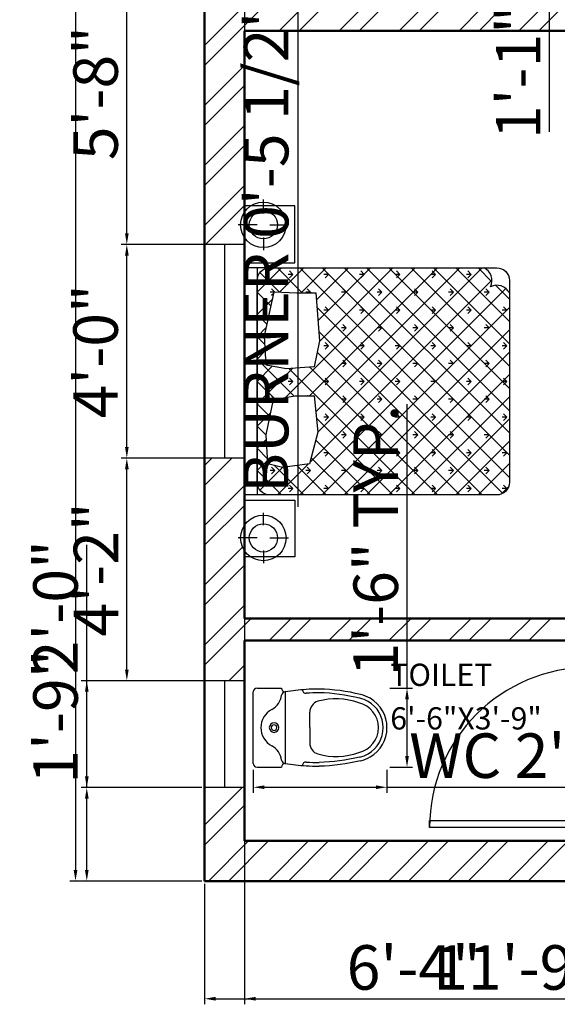
# Model space of a CAD drawing. Units: inches. Extents: x 3824 to 4289, y 1731 to 2259.
# Tile 1 of 5: x 3831 to 3952, y 1731 to 1952. Entities that reach past the tile are written whole.
import ezdxf

# ---------------------------------------------------------------- set-up
doc = ezdxf.new("R2010")
doc.units = ezdxf.units.IN
for name, color, linetype, lineweight in [('A-ANNO-DIMS', 2, 'Continuous', 18), ('A-AREA-IDEN', 2, 'Continuous', 18), ('A-FLOR-FIXT', 9, 'Continuous', 18), ('A-FURN', 9, 'Continuous', 18), ('DOOR', 6, 'Continuous', 25), ('WALL', 20, 'Continuous', 50), ('WINDOW', 4, 'Continuous', 25)]:
    doc.layers.add(name, color=color, linetype=linetype, lineweight=lineweight)
doc.layers.add('A-WALL-PATT', color=251, linetype='Continuous', lineweight=13, true_color=0x636466)
for name, color, linetype in [('GIUONG', 70, 'Continuous'), ('NOI THAT', 42, 'Continuous'), ('THIET-BI', 21, 'Continuous')]:
    doc.layers.add(name, color=color, linetype=linetype)
doc.styles.get("Standard").update_dxf_attribs({"font": 'arial.ttf'})
doc.dimstyles.new('ISO-25', dxfattribs={"dimtxt": 10, "dimasz": 2.5, "dimexe": 1.25, "dimexo": 0.625, "dimtad": 1, "dimdec": 1, "dimlunit": 3, "dimtxsty": 'Standard', "dimcen": 2.5, "dimadec": 0, "dimazin": 0, "dimtfac": 1, "dimtdec": 1, "dimtmove": 0, "dimatfit": 3, "dimfxl": 1, "dimarcsym": 0})

# ---------------------------------------------------------------- blocks, each defined once
blk = doc.blocks.new('A$C7C314EA1')
at = {"layer": 'THIET-BI'}
for p, q in [((20, 420), (150, 420)), ((0, 20), (0, 400)), ((170, 400), (170, 20)), ((300, 210), (300, 292.2)), ((300, 210), (300, 127.8)), ((20, 0), (150, 0)), ((20, 0), (150, 0))]:
    blk.add_line(p, q, dxfattribs=at)
for points in [[(279.9, 412.5, 0.02753), (170, 400, 0.02753)], [(564.9, 366.1, 0.054905), (349.5, 395, 0.054905)], [(569.7, 385.6, 0.054905), (350, 415, 0.054905)], [(300, 210), (300, 290, 0.704392)], [(300, 210), (300, 130, -0.704392)], [(564.9, 53.9, -0.054905), (349.5, 25, -0.054905)], [(170, 20, 0.02753), (279.9, 7.5, 0.02753)], [(569.7, 34.4, -0.054905), (350, 5, -0.054905)]]:
    blk.add_lwpolyline(points, format="xyb", dxfattribs=at)
for centre, radius, start, end in [((20, 400), 20, 90, 180), ((170, 420), 20, 180, 270), ((51, 395.2), 100, 298.1382, 352.7323), ((170, 380), 20, 90, 172.7323), ((279.9, 412.5), 20, 184.5905, 273.8823), ((350, -585), 1000, 90, 94.0204), ((350, -585), 980, 90, 94.0204), ((530, 210), 160, 60, 77.2425), ((530, 210), 180, 60, 77.2425), ((360, 292.2), 60, 105.9249, 180), ((439, 15.2), 348.1, 69.701, 105.9249), ((530, 210), 135, 0, 77.2425), ((530, 210), 160, 0, 60), ((530, 210), 180, 0, 60), ((150, 210), 110, 118.1382, 180), ((150, 210), 110, 180, 241.8618), ((150, 210), 110, 180, 241.8618), ((110, 210), 25, 0, 180), ((110, 210), 25, 0, 180), ((110, 210), 25, 180, 0), ((110, 210), 25, 180, 0), ((110, 210), 15, 0, 180), ((110, 210), 15, 0, 180), ((110, 210), 15, 180, 0), ((110, 210), 15, 180, 0), ((530, 210), 135, 282.7575, 0), ((530, 210), 160, 300, 0), ((530, 210), 180, 300, 0), ((51, 24.8), 100, 7.2677, 61.8618), ((51, 24.8), 100, 7.2677, 61.8618), ((360, 127.8), 60, 180, 254.0751), ((439, 404.8), 348.1, 254.0751, 290.299), ((530, 210), 160, 282.7575, 300), ((530, 210), 180, 282.7575, 300), ((20, 20), 20, 180, 270), ((170, 0), 20, 90, 180), ((170, 40), 20, 187.2677, 270), ((170, 40), 20, 187.2677, 270), ((279.9, 7.5), 20, 86.1177, 175.4095), ((350, 1005), 1000, 265.9796, 270), ((350, 1005), 980, 265.9796, 270)]:
    blk.add_arc(centre, radius, start, end, dxfattribs=at)
blk = doc.blocks.new('*U2')
for p, q in [((0, 0), (0, -6)), ((40, 0), (40, -6))]:
    blk.add_line(p, q)
blk.add_lwpolyline([(0, 0), (0, 40), (1.75, 40), (1.75, 0)], close=True)
blk.add_arc((0, 0), 40, 0, 90)
blk = doc.blocks.new('*X4')
at = {"color": 0}
for p, q in [((0, 0), (0, 0)), ((-565.7, 0), (-565.7, 0)), ((-565.7, 0), (-565.7, 0)), ((-282.8, 0), (-282.8, 0)), ((-282.8, 0), (-282.8, 0)), ((282.8, 0), (282.8, 0)), ((565.7, 0), (565.7, 0)), ((-707.1, -141.4), (-733.6, -114.9)), ((-707.1, -141.4), (-707.1, -103.9)), ((-707.1, -141.4), (-680.6, -114.9)), ((-156.4, -126.5), (-167.9, -114.9)), ((-141.4, -141.4), (-142.5, -140.4)), ((-141.4, -141.4), (-141.4, -103.9)), ((-141.4, -141.4), (-114.9, -114.9)), ((119.7, -119.7), (114.9, -114.9)), ((699.4, -133.7), (680.6, -114.9)), ((707.1, -135.4), (707.1, -103.9)), ((710, -138.6), (733.6, -114.9)), ((-848.5, -282.8), (-875, -256.3)), ((-848.5, -282.8), (-848.5, -245.3)), ((-848.5, -282.8), (-822, -256.3)), ((0, -282.8), (-26.5, -256.3)), ((0, -282.8), (0, -245.3)), ((0, -282.8), (26.5, -256.3)), ((848.5, -282.8), (822, -256.3)), ((848.5, -282.8), (848.5, -245.3)), ((848.5, -282.8), (875, -256.3)), ((-707.1, -424.3), (-707.1, -386.8)), ((707.1, -424.3), (707.1, -386.8)), ((-707.1, -424.3), (-733.6, -397.7)), ((-707.1, -424.3), (-680.6, -397.7)), ((-115.7, -398.5), (-114.9, -397.7)), ((707.1, -424.3), (702.9, -420)), ((707.1, -424.3), (733.6, -397.7)), ((-848.5, -565.7), (-875, -539.2)), ((-848.5, -565.7), (-848.5, -528.2)), ((-848.5, -565.7), (-822, -539.2)), ((-565.7, -565.7), (-592.2, -539.2)), ((-565.7, -565.7), (-565.7, -528.2)), ((-565.7, -565.7), (-539.2, -539.2)), ((-282.8, -565.7), (-309.4, -539.2)), ((-282.8, -565.7), (-282.8, -528.2)), ((-282.8, -565.7), (-256.3, -539.2)), ((0, -565.7), (-26.5, -539.2)), ((0, -565.7), (0, -528.2)), ((0, -565.7), (26.5, -539.2)), ((282.8, -565.7), (256.3, -539.2)), ((282.8, -565.7), (282.8, -528.2)), ((282.8, -565.7), (309.4, -539.2)), ((565.7, -565.7), (539.2, -539.2)), ((565.7, -565.7), (565.7, -528.2)), ((565.7, -565.7), (592.2, -539.2)), ((848.5, -565.7), (822, -539.2)), ((848.5, -565.7), (848.5, -528.2)), ((848.5, -565.7), (875, -539.2)), ((-707.1, -707.1), (-733.6, -680.6)), ((-707.1, -707.1), (-707.1, -669.6)), ((-707.1, -707.1), (-680.6, -680.6)), ((-424.3, -707.1), (-450.8, -680.6)), ((-424.3, -707.1), (-424.3, -669.6)), ((-424.3, -707.1), (-397.7, -680.6)), ((-141.4, -707.1), (-167.9, -680.6)), ((-141.4, -707.1), (-141.4, -669.6)), ((-141.4, -707.1), (-114.9, -680.6)), ((141.4, -707.1), (114.9, -680.6)), ((141.4, -707.1), (141.4, -669.6)), ((141.4, -707.1), (167.9, -680.6)), ((424.3, -707.1), (397.7, -680.6)), ((424.3, -707.1), (424.3, -669.6)), ((424.3, -707.1), (450.8, -680.6)), ((707.1, -707.1), (680.6, -680.6)), ((707.1, -707.1), (707.1, -669.6)), ((707.1, -707.1), (733.6, -680.6)), ((-848.5, -848.5), (-875, -822)), ((-848.5, -848.5), (-848.5, -811)), ((-848.5, -848.5), (-822, -822)), ((-565.7, -848.5), (-592.2, -822)), ((-565.7, -848.5), (-565.7, -811)), ((-565.7, -848.5), (-539.2, -822)), ((-282.8, -848.5), (-309.4, -822)), ((-282.8, -848.5), (-282.8, -811)), ((-282.8, -848.5), (-256.3, -822)), ((0, -848.5), (-26.5, -822)), ((0, -848.5), (0, -811)), ((0, -848.5), (26.5, -822)), ((282.8, -848.5), (256.3, -822)), ((282.8, -848.5), (282.8, -811)), ((282.8, -848.5), (309.4, -822)), ((565.7, -848.5), (539.2, -822)), ((565.7, -848.5), (565.7, -811)), ((565.7, -848.5), (592.2, -822)), ((848.5, -848.5), (822, -822)), ((848.5, -848.5), (848.5, -811)), ((848.5, -848.5), (875, -822)), ((-707.1, -989.9), (-733.6, -963.4)), ((-707.1, -989.9), (-707.1, -952.4)), ((-707.1, -989.9), (-680.6, -963.4)), ((-424.3, -989.9), (-450.8, -963.4)), ((-424.3, -989.9), (-424.3, -952.4)), ((-424.3, -989.9), (-397.7, -963.4)), ((-141.4, -989.9), (-167.9, -963.4)), ((-141.4, -989.9), (-141.4, -952.4)), ((-141.4, -989.9), (-114.9, -963.4)), ((141.4, -989.9), (114.9, -963.4)), ((141.4, -989.9), (141.4, -952.4)), ((141.4, -989.9), (167.9, -963.4)), ((424.3, -989.9), (397.7, -963.4)), ((424.3, -989.9), (424.3, -952.4)), ((424.3, -989.9), (450.8, -963.4)), ((707.1, -989.9), (680.6, -963.4)), ((707.1, -989.9), (707.1, -952.4)), ((707.1, -989.9), (733.6, -963.4)), ((-848.5, -1131.4), (-875, -1104.9)), ((-848.5, -1131.4), (-848.5, -1093.9)), ((-848.5, -1131.4), (-822, -1104.9)), ((-565.7, -1131.4), (-592.2, -1104.9)), ((-565.7, -1131.4), (-565.7, -1093.9)), ((-565.7, -1131.4), (-539.2, -1104.9)), ((-282.8, -1131.4), (-309.4, -1104.9)), ((-282.8, -1131.4), (-282.8, -1093.9)), ((-282.8, -1131.4), (-256.3, -1104.9)), ((0, -1131.4), (-26.5, -1104.9)), ((0, -1131.4), (0, -1093.9)), ((0, -1131.4), (26.5, -1104.9)), ((282.8, -1131.4), (256.3, -1104.9)), ((282.8, -1131.4), (282.8, -1093.9)), ((282.8, -1131.4), (309.4, -1104.9)), ((565.7, -1131.4), (539.2, -1104.9)), ((565.7, -1131.4), (565.7, -1093.9)), ((565.7, -1131.4), (592.2, -1104.9)), ((848.5, -1131.4), (822, -1104.9)), ((848.5, -1131.4), (848.5, -1093.9)), ((848.5, -1131.4), (875, -1104.9)), ((-707.1, -1272.8), (-733.6, -1246.3)), ((-707.1, -1272.8), (-707.1, -1235.3)), ((-707.1, -1272.8), (-680.6, -1246.3)), ((-424.3, -1272.8), (-450.8, -1246.3)), ((-424.3, -1272.8), (-424.3, -1235.3)), ((-424.3, -1272.8), (-397.7, -1246.3)), ((-141.4, -1272.8), (-167.9, -1246.3)), ((-141.4, -1272.8), (-141.4, -1235.3)), ((-141.4, -1272.8), (-114.9, -1246.3)), ((141.4, -1272.8), (114.9, -1246.3)), ((141.4, -1272.8), (141.4, -1235.3)), ((141.4, -1272.8), (167.9, -1246.3)), ((424.3, -1272.8), (397.7, -1246.3)), ((424.3, -1272.8), (424.3, -1235.3)), ((424.3, -1272.8), (450.8, -1246.3)), ((707.1, -1272.8), (680.6, -1246.3)), ((707.1, -1272.8), (707.1, -1235.3)), ((707.1, -1272.8), (733.6, -1246.3)), ((-848.5, -1414.2), (-875, -1387.7)), ((-848.5, -1414.2), (-848.5, -1376.7)), ((-848.5, -1414.2), (-822, -1387.7)), ((-565.7, -1414.2), (-592.2, -1387.7)), ((-565.7, -1414.2), (-565.7, -1376.7)), ((-565.7, -1414.2), (-539.2, -1387.7)), ((-282.8, -1414.2), (-309.4, -1387.7)), ((-282.8, -1414.2), (-282.8, -1376.7)), ((-282.8, -1414.2), (-256.3, -1387.7)), ((0, -1414.2), (-26.5, -1387.7)), ((0, -1414.2), (0, -1376.7)), ((0, -1414.2), (26.5, -1387.7)), ((282.8, -1414.2), (256.3, -1387.7)), ((282.8, -1414.2), (282.8, -1376.7)), ((282.8, -1414.2), (309.4, -1387.7)), ((565.7, -1414.2), (539.2, -1387.7)), ((565.7, -1414.2), (565.7, -1376.7)), ((565.7, -1414.2), (592.2, -1387.7)), ((848.5, -1414.2), (822, -1387.7)), ((848.5, -1414.2), (848.5, -1376.7)), ((848.5, -1414.2), (875, -1387.7)), ((-707.1, -1555.6), (-733.6, -1529.1)), ((-707.1, -1555.6), (-707.1, -1518.1)), ((-707.1, -1555.6), (-680.6, -1529.1)), ((-424.3, -1555.6), (-450.8, -1529.1)), ((-424.3, -1555.6), (-424.3, -1518.1)), ((-424.3, -1555.6), (-397.7, -1529.1)), ((-141.4, -1555.6), (-167.9, -1529.1)), ((-141.4, -1555.6), (-141.4, -1518.1)), ((-141.4, -1555.6), (-114.9, -1529.1)), ((141.4, -1555.6), (114.9, -1529.1)), ((141.4, -1555.6), (141.4, -1518.1)), ((141.4, -1555.6), (167.9, -1529.1)), ((424.3, -1555.6), (397.7, -1529.1)), ((424.3, -1555.6), (424.3, -1518.1)), ((424.3, -1555.6), (450.8, -1529.1)), ((707.1, -1555.6), (680.6, -1529.1)), ((707.1, -1555.6), (707.1, -1518.1)), ((707.1, -1555.6), (733.6, -1529.1)), ((-848.5, -1697.1), (-875, -1670.5)), ((-848.5, -1697.1), (-848.5, -1659.6)), ((-848.5, -1697.1), (-822, -1670.5)), ((-565.7, -1697.1), (-592.2, -1670.5)), ((-565.7, -1697.1), (-565.7, -1659.6)), ((-565.7, -1697.1), (-539.2, -1670.5)), ((-282.8, -1697.1), (-309.4, -1670.5)), ((-282.8, -1697.1), (-282.8, -1659.6)), ((-282.8, -1697.1), (-256.3, -1670.5)), ((0, -1697.1), (-26.5, -1670.5)), ((0, -1697.1), (0, -1659.6)), ((0, -1697.1), (26.5, -1670.5)), ((282.8, -1697.1), (256.3, -1670.5)), ((282.8, -1697.1), (282.8, -1659.6)), ((282.8, -1697.1), (309.4, -1670.5)), ((565.7, -1697.1), (539.2, -1670.5)), ((565.7, -1697.1), (565.7, -1659.6)), ((565.7, -1697.1), (592.2, -1670.5)), ((848.5, -1697.1), (822, -1670.5)), ((848.5, -1697.1), (848.5, -1659.6)), ((848.5, -1697.1), (875, -1670.5)), ((-707.1, -1838.5), (-733.6, -1812)), ((-707.1, -1838.5), (-707.1, -1801)), ((-707.1, -1838.5), (-680.6, -1812)), ((-424.3, -1838.5), (-450.8, -1812)), ((-424.3, -1838.5), (-424.3, -1801)), ((-424.3, -1838.5), (-397.7, -1812)), ((-141.4, -1838.5), (-167.9, -1812)), ((-141.4, -1838.5), (-141.4, -1801)), ((-141.4, -1838.5), (-114.9, -1812)), ((141.4, -1838.5), (114.9, -1812)), ((141.4, -1838.5), (141.4, -1801)), ((141.4, -1838.5), (167.9, -1812)), ((424.3, -1838.5), (397.7, -1812)), ((424.3, -1838.5), (424.3, -1801)), ((424.3, -1838.5), (450.8, -1812)), ((707.1, -1838.5), (680.6, -1812)), ((707.1, -1838.5), (707.1, -1801)), ((707.1, -1838.5), (733.6, -1812)), ((-848.5, -1979.9), (-848.5, -1942.4)), ((-565.7, -1979.9), (-565.7, -1942.4)), ((-282.8, -1979.9), (-282.8, -1942.4)), ((0, -1979.9), (0, -1942.4)), ((282.8, -1979.9), (282.8, -1942.4)), ((565.7, -1979.9), (565.7, -1942.4)), ((-848.5, -1979.9), (-875, -1953.4)), ((-848.5, -1979.9), (-822, -1953.4)), ((-565.7, -1979.9), (-592.2, -1953.4)), ((-565.7, -1979.9), (-539.2, -1953.4)), ((-282.8, -1979.9), (-309.4, -1953.4)), ((-282.8, -1979.9), (-256.3, -1953.4)), ((0, -1979.9), (-26.5, -1953.4)), ((0, -1979.9), (26.5, -1953.4)), ((282.8, -1979.9), (256.3, -1953.4)), ((282.8, -1979.9), (309.4, -1953.4)), ((565.7, -1979.9), (539.2, -1953.4)), ((565.7, -1979.9), (592.2, -1953.4))]:
    blk.add_line(p, q, dxfattribs=at)
blk = doc.blocks.new('*X3')
at = {"color": 0}
for p, q in [((-900, -192.9), (-707.1, 0)), ((-623.2, -83.9), (-707.1, 0)), ((-613.7, -83.3), (-530.3, 0)), ((-456.8, -73.5), (-530.3, 0)), ((-425.1, -71.6), (-353.6, 0)), ((-245.3, -108.2), (-353.6, 0)), ((-278.3, -101.5), (-176.8, 0)), ((103, -279.8), (-176.8, 0)), ((-142.2, -142.2), (0, 0)), ((-116.9, -293.7), (176.8, 0)), ((119.7, -119.7), (0, 0)), ((241.2, -64.5), (176.8, 0)), ((292.3, -61.3), (353.6, 0)), ((425.9, -72.3), (353.6, 0)), ((452.1, -78.2), (530.3, 0)), ((653.8, -123.5), (530.3, 0)), ((596.5, -110.6), (707.1, 0)), ((900, -192.9), (707.1, 0)), ((-682.9, -201), (-862.2, -21.7)), ((708.5, -175.4), (862.2, -21.7)), ((-900, -369.7), (-666.9, -136.6)), ((-655.7, -405), (-900, -160.7)), ((900, -1253.6), (-128.3, -225.2)), ((702.9, -357.8), (900, -160.7)), ((900, -369.7), (708.4, -178.1)), ((-900, -1253.6), (101.2, -252.3)), ((-900, -546.4), (-667.8, -314.2)), ((735.1, -1972.5), (-900, -337.4)), ((-762.6, -2000), (900, -337.4)), ((900, -546.4), (702.9, -349.3)), ((-900, -1430.3), (111.9, -418.4)), ((-900, -723.2), (-605.3, -428.5)), ((-900, -900), (-464.7, -464.7)), ((801.1, -1861.8), (-641.4, -419.2)), ((900, -1607.1), (-242.6, -464.5)), ((900, -1430.3), (-115.7, -414.7)), ((-900, -1076.8), (-292.7, -469.5)), ((-900, -1607.1), (231.1, -476)), ((-900, -1783.9), (394.4, -489.4)), ((585.8, -2000), (-900, -514.2)), ((-887.6, -1948.2), (585.6, -475)), ((-585.8, -2000), (900, -514.2)), ((900, -1783.9), (-403.5, -480.4)), ((900, -1076.8), (317, -493.8)), ((900, -900), (482.8, -482.8)), ((900, -723.2), (647.2, -470.4)), ((409, -2000), (-900, -691)), ((-409, -2000), (900, -691)), ((232.2, -2000), (-900, -867.8)), ((-232.2, -2000), (900, -867.8)), ((55.5, -2000), (-900, -1044.5)), ((-55.5, -2000), (900, -1044.5)), ((-121.3, -2000), (-900, -1221.3)), ((121.3, -2000), (900, -1221.3)), ((-298.1, -2000), (-900, -1398.1)), ((298.1, -2000), (900, -1398.1)), ((-474.9, -2000), (-900, -1574.9)), ((474.9, -2000), (900, -1574.9)), ((-651.7, -2000), (-900, -1751.7)), ((790.3, -1861.4), (900, -1751.7)), ((-834.6, -1993.8), (-893.8, -1934.6)), ((651.7, -2000), (761.4, -1890.3))]:
    blk.add_line(p, q, dxfattribs=at)
blk = doc.blocks.new('A$C190D2546')
at = {"layer": 'GIUONG'}
for points in [[(786.7, 1584.1), (758, 1799.3), (786.7, 1914.1), (1016.5, 1928.5), (1296.5, 1871.1), (1325.2, 1698.9), (1325.2, 1548.2), (1038, 1519.5)], [(1555, 1548.2), (1540.6, 1770.6), (1569.4, 1928.5), (1799.1, 1942.8), (2151, 1863.9), (2143.8, 1684.5), (2143.8, 1533.8), (1763.2, 1505.1)]]:
    blk.add_lwpolyline(points, close=True, dxfattribs=at)
for centre, radius in [((200, 1950.7), 180.3), ((2681.8, 1950.7), 180.3), ((200, 1950.7), 111.8), ((2681.8, 1950.7), 111.8)]:
    blk.add_circle(centre, radius, dxfattribs=at)
at = {"layer": 'NOI THAT'}
for p, q in [((200, 2000.7), (200, 2150.7)), ((2681.8, 2000.7), (2681.8, 2150.7)), ((540.9, 2100), (2340.9, 2100)), ((540.9, 1880.7), (540.9, 2100)), ((2340.9, 1880.7), (2340.9, 2100)), ((2340.9, 2000), (540.9, 2000)), ((100, 1950.7), (0, 1950.7)), ((200, 1900.7), (200, 1750.7)), ((300, 1950.7), (400, 1950.7)), ((2581.8, 1950.7), (2481.8, 1950.7)), ((2681.8, 1900.7), (2681.8, 1750.7)), ((2781.8, 1950.7), (2881.8, 1950.7))]:
    blk.add_line(p, q, dxfattribs=at)
for points in [[(500, 2100.7), (500, 1700.7), (50, 1700.7), (50, 2100.7)], [(2381.8, 2100.7), (2381.8, 1700.7), (2831.8, 1700.7), (2831.8, 2100.7)]]:
    blk.add_lwpolyline(points, close=True, dxfattribs=at)
blk.add_lwpolyline([(640.9, 2000), (2240.9, 2000, -0.414214), (2340.9, 1900), (2340.9, 100, -0.414214), (2240.9, 0), (640.9, 0, -0.414214), (540.9, 100), (540.9, 1900, -0.414214)], format="xyb", close=True, dxfattribs=at)
for centre, start, end in [((2240.9, 250), 243.43495, 333.43495), ((2090.9, 100), 296.56505, 26.56505)]:
    blk.add_arc(centre, 111.8, start, end, dxfattribs=at)
for name in ['*X3', '*X4']:
    blk.add_blockref(name, (1440.9, 2000), dxfattribs=at)
blk = doc.blocks.new('*D12')
at = {"layer": 'A-ANNO-DIMS', "color": 0, "lineweight": -2, "transparency": 16777216}
for p, q in [((3871.93, 2202.62), (3842.32, 2202.62)), ((3843.57, 2200.12), (3843.57, 1761.12)), ((3871.93, 1758.62), (3842.32, 1758.62))]:
    blk.add_line(p, q, dxfattribs=at)
at = {"layer": 'A-ANNO-DIMS', "color": 0, "transparency": 16777216}
for points in [[(3843.15, 2200.12), (3843.99, 2200.12), (3843.57, 2202.62)], [(3843.15, 1761.12), (3843.99, 1761.12), (3843.57, 1758.62)]]:
    blk.add_solid(points, dxfattribs=at)
at = {"layer": 'Defpoints', "color": 0, "transparency": 16777216}
for p in [(3872.55, 2202.62), (3843.57, 1758.62), (3872.55, 1758.62)]:
    blk.add_point(p, dxfattribs=at)
at = {"layer": 'A-ANNO-DIMS', "color": 0, "transparency": 16777216, "insert": (3837.84, 1980.62), "char_height": 10, "attachment_point": 5, "rotation": 90}
blk.add_mtext("37'", dxfattribs=at)
blk = doc.blocks.new('*D16')
at = {"layer": 'A-ANNO-DIMS', "color": 0, "lineweight": -2, "transparency": 16777216}
for p, q in [((3883.53, 1783.56), (3883.53, 1778.43)), ((3913.57, 1783.56), (3913.57, 1778.43)), ((3886.03, 1779.68), (3911.07, 1779.68)), ((3913.57, 1779.68), (4005.84, 1779.68))]:
    blk.add_line(p, q, dxfattribs=at)
at = {"layer": 'A-ANNO-DIMS', "color": 0, "transparency": 16777216}
for points in [[(3886.03, 1780.1), (3886.03, 1779.27), (3883.53, 1779.68)], [(3911.07, 1780.1), (3911.07, 1779.27), (3913.57, 1779.68)]]:
    blk.add_solid(points, dxfattribs=at)
at = {"layer": 'Defpoints', "color": 0, "transparency": 16777216}
for p in [(3883.53, 1784.19), (3913.57, 1784.19), (3913.57, 1779.68)]:
    blk.add_point(p, dxfattribs=at)
at = {"layer": 'A-ANNO-DIMS', "color": 0, "transparency": 16777216, "insert": (3960.95, 1785.48), "char_height": 10, "attachment_point": 5}
blk.add_mtext('WC 2\'-6" TYP.', dxfattribs=at)
blk = doc.blocks.new('*D17')
at = {"layer": 'A-ANNO-DIMS', "color": 0, "lineweight": -2, "transparency": 16777216}
for p, q in [((3918.07, 1801.96), (3918.07, 1865.72)), ((3914.19, 1801.96), (3919.32, 1801.96)), ((3918.07, 1786.69), (3918.07, 1799.46)), ((3914.19, 1784.19), (3919.32, 1784.19))]:
    blk.add_line(p, q, dxfattribs=at)
at = {"layer": 'A-ANNO-DIMS', "color": 0, "transparency": 16777216}
for points in [[(3917.66, 1799.46), (3918.49, 1799.46), (3918.07, 1801.96)], [(3917.66, 1786.69), (3918.49, 1786.69), (3918.07, 1784.19)]]:
    blk.add_solid(points, dxfattribs=at)
at = {"layer": 'Defpoints', "color": 0, "transparency": 16777216}
for p in [(3913.57, 1801.96), (3918.07, 1801.96), (3913.57, 1784.19)]:
    blk.add_point(p, dxfattribs=at)
at = {"layer": 'A-ANNO-DIMS', "color": 0, "transparency": 16777216, "insert": (3912.34, 1835.09), "char_height": 10, "attachment_point": 5, "rotation": 90}
blk.add_mtext('1\'-6" TYP.', dxfattribs=at)
blk = doc.blocks.new('*D18')
at = {"layer": 'A-ANNO-DIMS', "color": 0, "lineweight": -2, "transparency": 16777216}
for p, q in [((3893.51, 2003.46), (3893.51, 2005.96)), ((3893.33, 2000.96), (3894.76, 2000.96)), ((3893.51, 2000.96), (3893.51, 1995.6)), ((3893.33, 1995.6), (3894.76, 1995.6)), ((3893.51, 1993.1), (3893.51, 1842.67))]:
    blk.add_line(p, q, dxfattribs=at)
at = {"layer": 'A-ANNO-DIMS', "color": 0, "transparency": 16777216}
for points in [[(3893.09, 2003.46), (3893.93, 2003.46), (3893.51, 2000.96)], [(3893.09, 1993.1), (3893.93, 1993.1), (3893.51, 1995.6)]]:
    blk.add_solid(points, dxfattribs=at)
at = {"layer": 'Defpoints', "color": 0, "transparency": 16777216}
for p in [(3892.71, 2000.96), (3892.71, 1995.6), (3893.51, 1995.6)]:
    blk.add_point(p, dxfattribs=at)
at = {"layer": 'A-ANNO-DIMS', "color": 0, "transparency": 16777216, "insert": (3887.71, 1916.64), "char_height": 10, "attachment_point": 5, "rotation": 90}
blk.add_mtext('BURNER 0\'-5 1/2" TYP.', dxfattribs=at)
blk = doc.blocks.new('*D23')
at = {"layer": 'A-ANNO-DIMS', "color": 0, "lineweight": -2, "transparency": 16777216}
for p, q in [((3945.56, 1969.27), (3951.25, 1969.27)), ((3950, 1966.77), (3950, 1958.81)), ((3945.56, 1956.31), (3951.25, 1956.31)), ((3950, 1956.31), (3950, 1926.92))]:
    blk.add_line(p, q, dxfattribs=at)
at = {"layer": 'A-ANNO-DIMS', "color": 0, "transparency": 16777216}
for points in [[(3949.58, 1966.77), (3950.42, 1966.77), (3950, 1969.27)], [(3949.58, 1958.81), (3950.42, 1958.81), (3950, 1956.31)]]:
    blk.add_solid(points, dxfattribs=at)
at = {"layer": 'Defpoints', "color": 0, "transparency": 16777216}
for p in [(3944.93, 1969.27), (3944.93, 1956.31), (3950, 1956.31)]:
    blk.add_point(p, dxfattribs=at)
at = {"layer": 'A-ANNO-DIMS', "color": 0, "transparency": 16777216, "insert": (3944.36, 1940.36), "char_height": 10, "attachment_point": 5, "rotation": 90}
blk.add_mtext('1\'-1"', dxfattribs=at)
blk = doc.blocks.new('*D24')
at = {"layer": 'A-ANNO-DIMS', "color": 0, "lineweight": -2, "transparency": 16777216}
for p, q in [((3846.1, 1779.62), (3846.1, 1809.01)), ((3871.93, 1779.62), (3844.85, 1779.62)), ((3846.1, 1761.12), (3846.1, 1777.12)), ((3871.93, 1758.62), (3844.85, 1758.62))]:
    blk.add_line(p, q, dxfattribs=at)
at = {"layer": 'A-ANNO-DIMS', "color": 0, "transparency": 16777216}
for points in [[(3845.69, 1777.12), (3846.52, 1777.12), (3846.1, 1779.62)], [(3845.69, 1761.12), (3846.52, 1761.12), (3846.1, 1758.62)]]:
    blk.add_solid(points, dxfattribs=at)
at = {"layer": 'Defpoints', "color": 0, "transparency": 16777216}
for p in [(3846.1, 1779.62), (3872.55, 1779.62), (3872.55, 1758.62)]:
    blk.add_point(p, dxfattribs=at)
at = {"layer": 'A-ANNO-DIMS', "color": 0, "transparency": 16777216, "insert": (3840.37, 1795.56), "char_height": 10, "attachment_point": 5, "rotation": 90}
blk.add_mtext('1\'-9"', dxfattribs=at)
blk = doc.blocks.new('*D25')
at = {"layer": 'A-ANNO-DIMS', "color": 0, "lineweight": -2, "transparency": 16777216}
for p, q in [((3846.1, 1803.62), (3846.1, 1834.12)), ((3871.93, 1803.62), (3844.85, 1803.62)), ((3846.1, 1782.12), (3846.1, 1801.12)), ((3871.93, 1779.62), (3844.85, 1779.62))]:
    blk.add_line(p, q, dxfattribs=at)
at = {"layer": 'A-ANNO-DIMS', "color": 0, "transparency": 16777216}
for points in [[(3845.69, 1801.12), (3846.52, 1801.12), (3846.1, 1803.62)], [(3845.69, 1782.12), (3846.52, 1782.12), (3846.1, 1779.62)]]:
    blk.add_solid(points, dxfattribs=at)
at = {"layer": 'Defpoints', "color": 0, "transparency": 16777216}
for p in [(3846.1, 1803.62), (3872.55, 1803.62), (3872.55, 1779.62)]:
    blk.add_point(p, dxfattribs=at)
at = {"layer": 'A-ANNO-DIMS', "color": 0, "transparency": 16777216, "insert": (3840.37, 1820.12), "char_height": 10, "attachment_point": 5, "rotation": 90}
blk.add_mtext('2\'-0"', dxfattribs=at)
blk = doc.blocks.new('*D26')
at = {"layer": 'A-ANNO-DIMS', "color": 0, "lineweight": -2, "transparency": 16777216}
for p, q in [((3880.93, 1853.62), (3853.85, 1853.62)), ((3855.1, 1806.12), (3855.1, 1851.12)), ((3880.93, 1803.62), (3853.85, 1803.62))]:
    blk.add_line(p, q, dxfattribs=at)
at = {"layer": 'A-ANNO-DIMS', "color": 0, "transparency": 16777216}
for points in [[(3854.69, 1851.12), (3855.52, 1851.12), (3855.1, 1853.62)], [(3854.69, 1806.12), (3855.52, 1806.12), (3855.1, 1803.62)]]:
    blk.add_solid(points, dxfattribs=at)
at = {"layer": 'Defpoints', "color": 0, "transparency": 16777216}
for p in [(3855.1, 1853.62), (3881.55, 1853.62), (3881.55, 1803.62)]:
    blk.add_point(p, dxfattribs=at)
at = {"layer": 'A-ANNO-DIMS', "color": 0, "transparency": 16777216, "insert": (3849.46, 1828.62), "char_height": 10, "attachment_point": 5, "rotation": 90}
blk.add_mtext('4\'-2"', dxfattribs=at)
blk = doc.blocks.new('*D27')
at = {"layer": 'A-ANNO-DIMS', "color": 0, "lineweight": -2, "transparency": 16777216}
for p, q in [((3880.93, 1901.62), (3853.85, 1901.62)), ((3855.1, 1856.12), (3855.1, 1899.12)), ((3880.93, 1853.62), (3853.85, 1853.62))]:
    blk.add_line(p, q, dxfattribs=at)
at = {"layer": 'A-ANNO-DIMS', "color": 0, "transparency": 16777216}
for points in [[(3854.69, 1899.12), (3855.52, 1899.12), (3855.1, 1901.62)], [(3854.69, 1856.12), (3855.52, 1856.12), (3855.1, 1853.62)]]:
    blk.add_solid(points, dxfattribs=at)
at = {"layer": 'Defpoints', "color": 0, "transparency": 16777216}
for p in [(3855.1, 1901.62), (3881.55, 1901.62), (3881.55, 1853.62)]:
    blk.add_point(p, dxfattribs=at)
at = {"layer": 'A-ANNO-DIMS', "color": 0, "transparency": 16777216, "insert": (3849.37, 1877.62), "char_height": 10, "attachment_point": 5, "rotation": 90}
blk.add_mtext('4\'-0"', dxfattribs=at)
blk = doc.blocks.new('*D28')
at = {"layer": 'A-ANNO-DIMS', "color": 0, "lineweight": -2, "transparency": 16777216}
for p, q in [((3880.93, 1969.62), (3853.85, 1969.62)), ((3855.1, 1904.12), (3855.1, 1967.12)), ((3880.93, 1901.62), (3853.85, 1901.62))]:
    blk.add_line(p, q, dxfattribs=at)
at = {"layer": 'A-ANNO-DIMS', "color": 0, "transparency": 16777216}
for points in [[(3854.69, 1967.12), (3855.52, 1967.12), (3855.1, 1969.62)], [(3854.69, 1904.12), (3855.52, 1904.12), (3855.1, 1901.62)]]:
    blk.add_solid(points, dxfattribs=at)
at = {"layer": 'Defpoints', "color": 0, "transparency": 16777216}
for p in [(3855.1, 1969.62), (3881.55, 1969.62), (3881.55, 1901.62)]:
    blk.add_point(p, dxfattribs=at)
at = {"layer": 'A-ANNO-DIMS', "color": 0, "transparency": 16777216, "insert": (3849.37, 1935.62), "char_height": 10, "attachment_point": 5, "rotation": 90}
blk.add_mtext('5\'-8"', dxfattribs=at)
blk = doc.blocks.new('*D38')
at = {"layer": 'A-ANNO-DIMS', "color": 0, "lineweight": -2, "transparency": 16777216}
for p, q in [((3872.55, 1757.99), (3872.55, 1730.92)), ((4013.55, 1757.99), (4013.55, 1730.92)), ((3875.05, 1732.17), (4011.05, 1732.17))]:
    blk.add_line(p, q, dxfattribs=at)
at = {"layer": 'A-ANNO-DIMS', "color": 0, "transparency": 16777216}
for points in [[(3875.05, 1732.59), (3875.05, 1731.75), (3872.55, 1732.17)], [(4011.05, 1732.59), (4011.05, 1731.75), (4013.55, 1732.17)]]:
    blk.add_solid(points, dxfattribs=at)
at = {"layer": 'Defpoints', "color": 0, "transparency": 16777216}
for p in [(3872.55, 1758.62), (4013.55, 1758.62), (4013.55, 1732.17)]:
    blk.add_point(p, dxfattribs=at)
at = {"layer": 'A-ANNO-DIMS', "color": 0, "transparency": 16777216, "insert": (3943.05, 1737.9), "char_height": 10, "attachment_point": 5}
blk.add_mtext('11\'-9"', dxfattribs=at)
blk = doc.blocks.new('*D58')
at = {"layer": 'A-ANNO-DIMS', "color": 0, "lineweight": -2, "transparency": 16777216}
for p, q in [((3881.55, 1953.99), (3881.55, 1730.92)), ((3957.61, 1953.99), (3957.61, 1730.92)), ((3884.05, 1732.17), (3955.11, 1732.17))]:
    blk.add_line(p, q, dxfattribs=at)
at = {"layer": 'A-ANNO-DIMS', "color": 0, "transparency": 16777216}
for points in [[(3884.05, 1732.59), (3884.05, 1731.75), (3881.55, 1732.17)], [(3955.11, 1732.59), (3955.11, 1731.75), (3957.61, 1732.17)]]:
    blk.add_solid(points, dxfattribs=at)
at = {"layer": 'Defpoints', "color": 0, "transparency": 16777216}
for p in [(3881.55, 1954.62), (3957.61, 1954.62), (3957.61, 1732.17)]:
    blk.add_point(p, dxfattribs=at)
at = {"layer": 'A-ANNO-DIMS', "color": 0, "transparency": 16777216, "insert": (3919.58, 1737.9), "char_height": 10, "attachment_point": 5}
blk.add_mtext('6\'-4"', dxfattribs=at)

msp = doc.modelspace()

# ---------------------------------------------------------------- hatches: boundary and pattern name
at = {"layer": 'A-WALL-PATT'}
h = msp.add_hatch(dxfattribs=at)
h.set_pattern_fill('ANSI32', color=256)
h.paths.add_polyline_path([(4018.55, 1954.62), (3881.55, 1954.62), (3881.55, 1969.62), (3872.55, 1969.62), (3872.55, 1901.62), (3881.53, 1901.62), (3881.53, 1903.2, -0.148069), (3880.67, 1906.03, -0.148069), (3881.53, 1908.87), (3881.53, 1910.29), (3881.55, 1949.62), (4013.55, 1949.62), (4013.55, 1940.62), (4018.55, 1940.62)])
h = msp.add_hatch(dxfattribs=at)
h.set_pattern_fill('ANSI32', color=256)
h.paths.add_polyline_path([(3881.55, 1812.62), (3959.55, 1812.62), (3959.55, 1806.62), (3964.55, 1806.62), (3964.55, 1812.62), (3968.55, 1812.62), (3968.55, 1817.62), (3881.55, 1817.62), (3881.55, 1831.44), (3881.53, 1831.44), (3881.53, 1832.85, -0.148069), (3880.67, 1835.69, -0.148069), (3881.53, 1838.52), (3881.53, 1844.19), (3881.53, 1853.62), (3872.55, 1853.62), (3872.55, 1803.62), (3881.55, 1803.62)])
h = msp.add_hatch(dxfattribs=at)
h.set_pattern_fill('ANSI32', color=256)
h.paths.add_polyline_path([(4013.55, 1767.62), (3964.55, 1767.62), (3964.55, 1770.62), (3959.55, 1770.62), (3959.55, 1767.62), (3881.55, 1767.62), (3881.55, 1779.62), (3872.55, 1779.62), (3872.55, 1758.62), (4013.55, 1758.62)])

# ---------------------------------------------------------------- linework, layer by layer
at = {"layer": 'WALL'}
for p, q in [((3872.55, 2202.62), (3872.55, 1758.62)), ((3881.55, 1949.62), (4013.55, 1949.62)), ((3881.55, 1949.62), (3881.55, 1817.62)), ((3881.55, 1817.62), (3968.55, 1817.62)), ((3881.55, 1812.62), (3959.55, 1812.62)), ((3881.55, 1812.62), (3881.55, 1767.62)), ((3881.55, 1767.62), (3959.55, 1767.62)), ((3872.55, 1758.62), (4013.55, 1758.62))]:
    msp.add_line(p, q, dxfattribs=at)
at = {"layer": 'WINDOW'}
for p, q in [((3881.55, 1901.62), (3872.55, 1901.62)), ((3877.05, 1901.62), (3877.05, 1853.62)), ((3881.55, 1853.62), (3872.55, 1853.62)), ((3881.55, 1803.62), (3872.55, 1803.62)), ((3877.05, 1803.62), (3877.05, 1779.62)), ((3881.55, 1779.62), (3872.55, 1779.62))]:
    msp.add_line(p, q, dxfattribs=at)

# ---------------------------------------------------------------- block references
at = {"layer": 'A-FLOR-FIXT', "xscale": 0.042307961426094, "yscale": 0.042307961426094, "zscale": 0.042307961426094}
msp.add_blockref('A$C7C314EA1', (3883.53, 1784.19), dxfattribs=at)
at = {"layer": 'A-FURN', "xscale": 0.0283444227516291, "yscale": 0.0283444227516291, "zscale": 0.0283444227516291, "rotation": 90}
msp.add_blockref('A$C190D2546', (3941.08, 1830.02), dxfattribs=at)
at = {"layer": 'DOOR', "xscale": 0.9000000000000028, "yscale": 0.9000000000000028, "zscale": 0.9000000000000028, "rotation": 90.00000000000003}
msp.add_blockref('*U2', (3959.15, 1770.62), dxfattribs=at)

# ---------------------------------------------------------------- texts
at = {"layer": 'A-AREA-IDEN'}
for s, p in [('TOILET', (3914.31, 1802.44)), ('6\'-6"X3\'-9"', (3914.31, 1792.66))]:
    msp.add_text(s, height=5, dxfattribs=at).set_placement(p)

# ---------------------------------------------------------------- dimensions: what is measured, and where the dimension line sits
at = {"layer": 'A-ANNO-DIMS'}
for base, p1, p2, angle, override, picture, middle in [((3843.57, 1758.62), (3872.55, 2202.62), (3872.55, 1758.62), 90, {"dimclrd": 0, "dimclre": 0, "dimclrt": 0}, '*D12', (3837.84, 1980.62)), ((3855.1, 1969.62), (3881.55, 1901.62), (3881.55, 1969.62), 90, {"dimdec": 1, "dimlfac": 1, "dimrnd": 0, "dimzin": 1, "dimdsep": 46, "dimlunit": 4, "dimfrac": 2}, '*D28', (3849.37, 1935.62)), ((3950, 1956.31), (3944.93, 1969.27), (3944.93, 1956.31), 270, {"dimdec": 1, "dimlfac": 1, "dimrnd": 0, "dimzin": 1, "dimdsep": 46, "dimlunit": 4, "dimfrac": 2}, '*D23', (3944.36, 1940.36)), ((3855.1, 1901.62), (3881.55, 1853.62), (3881.55, 1901.62), 90, {"dimdec": 1, "dimlfac": 1, "dimrnd": 0, "dimzin": 1, "dimdsep": 46, "dimlunit": 4, "dimfrac": 2}, '*D27', (3849.37, 1877.62)), ((3855.1, 1853.62), (3881.55, 1803.62), (3881.55, 1853.62), 90, {"dimdec": 1, "dimlfac": 1, "dimrnd": 0, "dimzin": 1, "dimdsep": 46, "dimlunit": 4, "dimfrac": 2}, '*D26', (3849.46, 1828.62)), ((3846.1, 1803.62), (3872.55, 1779.62), (3872.55, 1803.62), 90, {"dimdec": 1, "dimlfac": 1, "dimrnd": 0, "dimzin": 1, "dimdsep": 46, "dimlunit": 4, "dimfrac": 2}, '*D25', (3840.37, 1820.12)), ((3846.1, 1779.62), (3872.55, 1758.62), (3872.55, 1779.62), 90, {"dimdec": 1, "dimlfac": 1, "dimrnd": 0, "dimzin": 1, "dimdsep": 46, "dimlunit": 4, "dimfrac": 2}, '*D24', (3840.37, 1795.56))]:
    dim = msp.add_linear_dim(base=base, p1=p1, p2=p2, angle=angle, dimstyle='ISO-25', override=override, dxfattribs=at)
    dim.commit()
    dim.dimension.update_dxf_attribs({"geometry": picture, "text_midpoint": middle})
for base, p1, p2, angle, text, picture, middle in [((3893.51, 1995.6), (3892.71, 2000.96), (3892.71, 1995.6), 270, 'BURNER <> TYP.', '*D18', (3887.71, 1916.64)), ((3918.07, 1801.96), (3913.57, 1784.19), (3913.57, 1801.96), 90, '<> TYP.', '*D17', (3912.34, 1835.09))]:
    dim = msp.add_linear_dim(base=base, p1=p1, p2=p2, angle=angle, text=text, dimstyle='ISO-25', override={"dimdec": 1, "dimlfac": 1, "dimrnd": 0, "dimzin": 1, "dimdsep": 46, "dimlunit": 4, "dimfrac": 2}, dxfattribs=at)
    dim.commit()
    dim.dimension.update_dxf_attribs({"geometry": picture, "text_midpoint": middle})
for base, p1, p2, picture, middle in [((3957.61, 1732.17), (3881.55, 1954.62), (3957.61, 1954.62), '*D58', (3919.58, 1737.9)), ((4013.55, 1732.17), (3872.55, 1758.62), (4013.55, 1758.62), '*D38', (3943.05, 1737.9))]:
    dim = msp.add_linear_dim(base=base, p1=p1, p2=p2, dimstyle='ISO-25', override={"dimdec": 1, "dimlfac": 1, "dimrnd": 0, "dimzin": 1, "dimdsep": 46, "dimlunit": 4, "dimfrac": 2}, dxfattribs=at)
    dim.commit()
    dim.dimension.update_dxf_attribs({"geometry": picture, "text_midpoint": middle})
dim = msp.add_linear_dim(base=(3913.57, 1779.68), p1=(3883.53, 1784.19), p2=(3913.57, 1784.19), text='WC <> TYP.', dimstyle='ISO-25', override={"dimdec": 1, "dimlfac": 1, "dimrnd": 0, "dimzin": 1, "dimdsep": 46, "dimlunit": 4, "dimfrac": 2}, dxfattribs=at)
dim.commit()
dim.dimension.update_dxf_attribs({"geometry": '*D16', "text_midpoint": (3960.95, 1785.48)})

doc.saveas('drawing.dxf')
